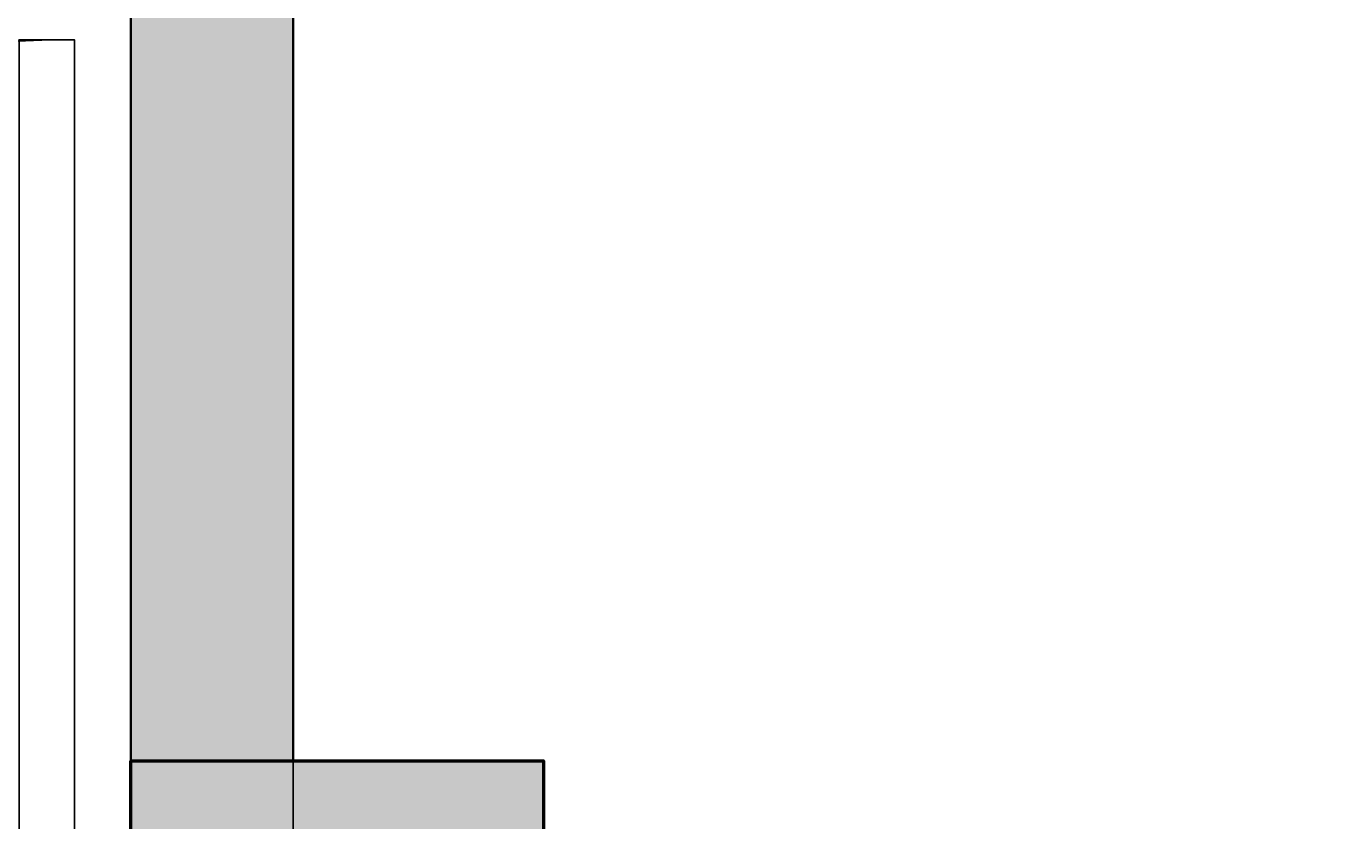
# Model space of a CAD drawing. Units: inches. Extents: x 1998 to 2588, y 1139 to 1977.
# Tile 29 of 134: x 2220 to 2257, y 1484 to 1506. Entities that reach past the tile are written whole.
import ezdxf

# ---------------------------------------------------------------- set-up
doc = ezdxf.new("R2010")
doc.units = ezdxf.units.IN
for name, color, linetype, lineweight in [('A-ANNO-DIMS', 2, 'Continuous', 18), ('A-COLS-PATT', 250, 'Continuous', 13), ('A-WALL-PATT', 252, 'Continuous', 13), ('COLUMN', 10, 'Continuous', 50), ('DOOR', 52, 'Continuous', 25), ('WALL', 200, 'Continuous', 35)]:
    doc.layers.add(name, color=color, linetype=linetype, lineweight=lineweight)
doc.styles.get("Standard").update_dxf_attribs({"font": 'arial.ttf'})
doc.dimstyles.get("Standard").update_dxf_attribs({"dimtxt": 0.18, "dimasz": 0.18, "dimexe": 0.18, "dimexo": 0.0625, "dimgap": 0.09, "dimtad": 0, "dimtih": 1, "dimtoh": 1, "dimdec": 4, "dimzin": 0, "dimdsep": 46, "dimtxsty": 'Standard', "dimcen": 0.09, "dimadec": 0, "dimazin": 0, "dimtfac": 1, "dimtdec": 4, "dimtofl": 0, "dimtmove": 0, "dimatfit": 3, "dimfxl": 1, "dimtolj": 1, "dimtzin": 0, "dimarcsym": 0})

# ---------------------------------------------------------------- blocks, each defined once
blk = doc.blocks.new('*U2')
blk.add_lwpolyline([(0, 0), (0, 40), (1.75, 40), (1.75, 0)], close=True)
blk.add_arc((0, 0), 40, 0, 90)
blk = doc.blocks.new('*D41')
at = {"layer": 'A-ANNO-DIMS', "color": 0, "lineweight": -2, "transparency": 16777216}
for p, q in [((2227.473, 1588.67), (2227.473, 1138.602)), ((2287.473, 1588.67), (2287.473, 1138.602)), ((2227.653, 1138.782), (2257.254, 1138.782)), ((2287.293, 1138.782), (2257.692, 1138.782))]:
    blk.add_line(p, q, dxfattribs=at)
at = {"layer": 'A-ANNO-DIMS', "color": 0, "transparency": 16777216}
for points in [[(2227.653, 1138.812), (2227.653, 1138.752), (2227.473, 1138.782)], [(2287.293, 1138.812), (2287.293, 1138.752), (2287.473, 1138.782)]]:
    blk.add_solid(points, dxfattribs=at)
at = {"layer": 'Defpoints', "color": 0, "transparency": 16777216}
for p in [(2227.473, 1588.732), (2287.473, 1588.732), (2287.473, 1138.782)]:
    blk.add_point(p, dxfattribs=at)
at = {"layer": 'A-ANNO-DIMS', "color": 0, "transparency": 16777216, "insert": (2257.473, 1138.782), "char_height": 0.18, "attachment_point": 5}
blk.add_mtext('\\A1;60', dxfattribs=at)

msp = doc.modelspace()

# ---------------------------------------------------------------- hatches: boundary and pattern name
at = {"layer": 'A-COLS-PATT'}
h = msp.add_hatch(color=256, dxfattribs=at)
h.dxf.hatch_style = 1
h.paths.add_polyline_path([(2099.4125, 1888.7324), (2087.9729, 1888.7324), (2087.9729, 1868.3278), (2099.4125, 1868.3278)])
h.paths.add_polyline_path([(2234.4125, 1888.7324), (2222.9729, 1888.7324), (2222.9729, 1868.3278), (2234.4125, 1868.3278)])
h.paths.add_polyline_path([(2341.4729, 1886.637), (2330.0332, 1886.637), (2330.0332, 1866.2324), (2341.4729, 1866.2324)])
h.paths.add_polyline_path([(2507.8006, 1882.7324), (2487.396, 1882.7324), (2487.396, 1871.2927), (2507.8006, 1871.2927)])
h.paths.add_polyline_path([(2510.9729, 1766.672), (2490.5682, 1766.672), (2490.5682, 1755.2324), (2510.9729, 1755.2324)])
h.paths.add_polyline_path([(2345.9729, 1759.7324), (2334.5332, 1759.7324), (2334.5332, 1739.3278), (2345.9729, 1739.3278)])
h.paths.add_polyline_path([(2234.4125, 1774.3318), (2222.9729, 1774.3318), (2222.9729, 1753.9272), (2234.4125, 1753.9272)])
h.paths.add_polyline_path([(2099.4125, 1775.637), (2087.9729, 1775.637), (2087.9729, 1755.2324), (2099.4125, 1755.2324)])
h.paths.add_polyline_path([(2098.0956, 1593.7241), (2077.691, 1593.7241), (2077.691, 1582.2845), (2098.0956, 1582.2845)])
h.paths.add_polyline_path([(2227.4729, 1604.637), (2216.0332, 1604.637), (2216.0332, 1584.2324), (2227.4729, 1584.2324)])
h.paths.add_polyline_path([(2345.9729, 1647.5211), (2334.5332, 1647.5211), (2334.5332, 1627.1165), (2345.9729, 1627.1165)])
h.paths.add_polyline_path([(2522.3775, 1641.2324), (2501.9729, 1641.2324), (2501.9729, 1629.7927), (2522.3775, 1629.7927)])
h.paths.add_polyline_path([(2522.3775, 1480.7324), (2501.9729, 1480.7324), (2501.9729, 1469.2927), (2522.3775, 1469.2927)])
h.paths.add_polyline_path([(2345.9729, 1488.5616), (2334.5332, 1488.5616), (2334.5332, 1468.1569), (2345.9729, 1468.1569)])
h.paths.add_polyline_path([(2234.4125, 1486.137), (2227.4729, 1486.137), (2227.4729, 1465.7324), (2234.4125, 1465.7324)])
h.paths.add_polyline_path([(2227.4729, 1486.137), (2222.9729, 1486.137), (2222.9729, 1465.7324), (2227.4729, 1465.7324)])
h.paths.add_polyline_path([(2108.3775, 1470.2324), (2087.9729, 1470.2324), (2087.9729, 1458.7927), (2108.3775, 1458.7927)])
h.paths.add_polyline_path([(2096.9729, 1365.5012), (2087.9729, 1365.5012), (2087.9729, 1345.0966), (2096.9729, 1345.0966)])
h.paths.add_polyline_path([(2087.9729, 1365.5012), (2085.5332, 1365.5012), (2085.5332, 1345.0966), (2087.9729, 1345.0966)])
h.paths.add_polyline_path([(2234.4125, 1285.137), (2222.9729, 1285.137), (2222.9729, 1264.7324), (2234.4125, 1264.7324)])
h.paths.add_polyline_path([(2345.9729, 1285.137), (2334.5332, 1285.137), (2334.5332, 1264.7324), (2345.9729, 1264.7324)])
h.paths.add_polyline_path([(2503.1458, 1240.172), (2482.7412, 1240.172), (2482.7412, 1228.7324), (2503.1458, 1228.7324)])
h.paths.add_polyline_path([(2510.9729, 1369.172), (2490.5682, 1369.172), (2490.5682, 1357.7324), (2510.9729, 1357.7324)])
at = {"layer": 'A-WALL-PATT'}
h = msp.add_hatch(color=256, dxfattribs=at)
h.dxf.hatch_style = 1
h.paths.add_polyline_path([(2222.9729, 1888.7324), (2099.4125, 1888.7324), (2099.4125, 1879.7324), (2222.9729, 1879.7324)])
h.paths.add_polyline_path([(2096.9729, 1868.3278), (2087.9729, 1868.3278), (2087.9729, 1775.637), (2096.9729, 1775.637)])
h.paths.add_polyline_path([(2227.4729, 1868.3278), (2222.9729, 1868.3278), (2222.9729, 1774.3318), (2227.4729, 1774.3318)])
h.paths.add_polyline_path([(2188.3019, 1759.7324), (2138.6074, 1759.7324), (2099.4125, 1759.7324), (2099.4125, 1755.2324), (2176.9729, 1755.2324), (2188.3019, 1755.2324)])
h.paths.add_polyline_path([(2087.9729, 1759.7324), (2059.4729, 1759.7324), (2059.4729, 1702.7324), (2087.9729, 1702.7324), (2087.9729, 1707.2324), (2063.9729, 1707.2324), (2063.9729, 1755.2324), (2087.9729, 1755.2324)])
h.paths.add_polyline_path([(2096.9729, 1755.2324), (2087.9729, 1755.2324), (2087.9729, 1707.2324), (2096.9729, 1707.2324)])
h.paths.add_polyline_path([(2187.0461, 1707.2324), (2105.9729, 1707.2324), (2096.9729, 1707.2324), (2087.9729, 1707.2324), (2087.9729, 1702.7324), (2105.9729, 1702.7324), (2114.9729, 1702.7324), (2187.0461, 1702.7324)])
h.paths.add_polyline_path([(2181.4729, 1719.2028), (2176.9729, 1719.2028), (2176.9729, 1707.2324), (2181.4729, 1707.2324)])
h.paths.add_polyline_path([(2216.0332, 1588.7324), (2114.9729, 1588.7324), (2105.9729, 1588.7324), (2105.9729, 1584.2324), (2216.0332, 1584.2324)])
h.paths.add_polyline_path([(2077.691, 1588.7324), (2061.4729, 1588.7324), (2061.4729, 1584.2324), (2077.691, 1584.2324)])
h.paths.add_polyline_path([(2105.9729, 1588.7324), (2098.0956, 1588.7324), (2098.0956, 1584.2324), (2105.9729, 1584.2324)])
h.paths.add_polyline_path([(2114.9729, 1596.2642), (2110.1012, 1596.2642), (2105.9729, 1596.2642), (2105.9729, 1588.7324), (2114.9729, 1588.7324)])
h.paths.add_polyline_path([(2114.9729, 1584.2324), (2105.9729, 1584.2324), (2105.9729, 1580.249), (2110.1012, 1580.249), (2114.9729, 1580.249)])
h.paths.add_polyline_path([(2114.9729, 1547.7716), (2110.1012, 1547.7716, -0.0318759), (2105.9729, 1548.035), (2105.9729, 1470.2324), (2108.3775, 1470.2324), (2108.3775, 1465.7324), (2186.2943, 1465.7324), (2186.2943, 1470.2324), (2114.9729, 1470.2324)])
h.paths.add_polyline_path([(2227.4729, 1584.2324), (2222.9729, 1584.2324), (2222.9729, 1486.137), (2227.4729, 1486.137)])
h.paths.add_polyline_path([(2295.4138, 1593.2324), (2227.4729, 1593.2324), (2227.4729, 1588.7324), (2295.4138, 1588.7324), (2295.4138, 1591.8729)])
h.paths.add_polyline_path([(2345.9729, 1627.1165), (2341.4729, 1627.1165), (2341.4729, 1593.2324), (2337.2869, 1593.2324), (2337.2869, 1591.8729), (2337.2869, 1588.7324), (2345.9729, 1588.7324)])
h.paths.add_polyline_path([(2291.9729, 1588.7324), (2287.4729, 1588.7324), (2287.4729, 1522.7324), (2291.9729, 1522.7324)])
h.paths.add_polyline_path([(2291.9729, 1522.7324), (2287.4729, 1522.7324), (2227.4729, 1522.7324), (2227.4729, 1518.2324), (2291.9729, 1518.2324)])
h.paths.add_polyline_path([(2295.7347, 1519.5919), (2295.7347, 1522.7324), (2291.9729, 1522.7324), (2291.9729, 1518.2324), (2295.7347, 1518.2324)])
h.paths.add_polyline_path([(2345.9729, 1522.7324), (2337.6078, 1522.7324), (2337.6078, 1519.5919), (2337.6078, 1518.2324), (2341.4729, 1518.2324), (2341.4729, 1488.5616), (2345.9729, 1488.5616)])
h.paths.add_polyline_path([(2345.9729, 1468.1569), (2341.4729, 1468.1569), (2341.4729, 1374.2324), (2227.4729, 1374.2324), (2227.4729, 1369.7324), (2345.9729, 1369.7324)])
h.paths.add_polyline_path([(2345.9729, 1369.7324), (2341.4729, 1369.7324), (2341.4729, 1362.2324), (2345.9729, 1362.2324)])
h.paths.add_polyline_path([(2345.9729, 1317.7324), (2345.9729, 1322.2324), (2341.4729, 1322.2324), (2341.4729, 1285.137), (2345.9729, 1285.137)], flags=17)
h.paths.add_polyline_path([(2356.2096, 1322.2324), (2345.9729, 1322.2324), (2345.9729, 1317.7324), (2356.2096, 1317.7324), (2356.2096, 1319.3088)], flags=17)
h.paths.add_polyline_path([(2393.9729, 1322.2324), (2375.6999, 1322.2324), (2375.6999, 1319.3088, -0.0202458), (2375.636, 1317.7324), (2393.9729, 1317.7324)], flags=17)
h.paths.add_polyline_path([(2398.4729, 1322.2324), (2393.9729, 1322.2324), (2393.9729, 1317.7324), (2393.9729, 1237.7324), (2345.9729, 1237.7324), (2345.9729, 1264.7324), (2341.4729, 1264.7324), (2341.4729, 1228.7324), (2393.9729, 1228.7324), (2482.7412, 1228.7324), (2482.7412, 1237.7324), (2398.4729, 1237.7324), (2398.4729, 1297.1029)])
h.paths.add_polyline_path([(2398.4729, 1362.2324), (2393.9729, 1362.2324), (2393.9729, 1357.7324), (2398.4729, 1357.7324)])
h.paths.add_polyline_path([(2345.9729, 1329.7549), (2341.4729, 1329.7549), (2341.4729, 1322.2324), (2345.9729, 1322.2324)])

# ---------------------------------------------------------------- linework, layer by layer
at = {"layer": 'COLUMN'}
msp.add_lwpolyline([(2222.9729, 1486.137), (2234.4125, 1486.137), (2234.4125, 1465.7324), (2222.9729, 1465.7324)], close=True, dxfattribs=at)
at = {"layer": 'WALL'}
for p, q in [((2227.4729, 1588.7324), (2227.4729, 1486.137)), ((2222.9729, 1584.2324), (2222.9729, 1486.137))]:
    msp.add_line(p, q, dxfattribs=at)

# ---------------------------------------------------------------- block references
at = {"layer": 'DOOR', "xscale": -0.877957807115804, "yscale": 0.877957807115804, "zscale": 0.877957807115804}
msp.add_blockref('*U2', (2221.4126, 1471.0001), dxfattribs=at)

# ---------------------------------------------------------------- dimensions: what is measured, and where the dimension line sits
at = {"layer": 'A-ANNO-DIMS'}
dim = msp.add_linear_dim(base=(2287.4729, 1138.7824), p1=(2227.4729, 1588.7324), p2=(2287.4729, 1588.7324), dimstyle='Standard', override={"dimdec": 0, "dimlfac": 1, "dimrnd": 0, "dimzin": 0, "dimdsep": 46, "dimlunit": 2}, dxfattribs=at)
dim.commit()
dim.dimension.update_dxf_attribs({"geometry": '*D41', "text_midpoint": (2257.4729, 1138.7824)})

doc.saveas('drawing.dxf')
